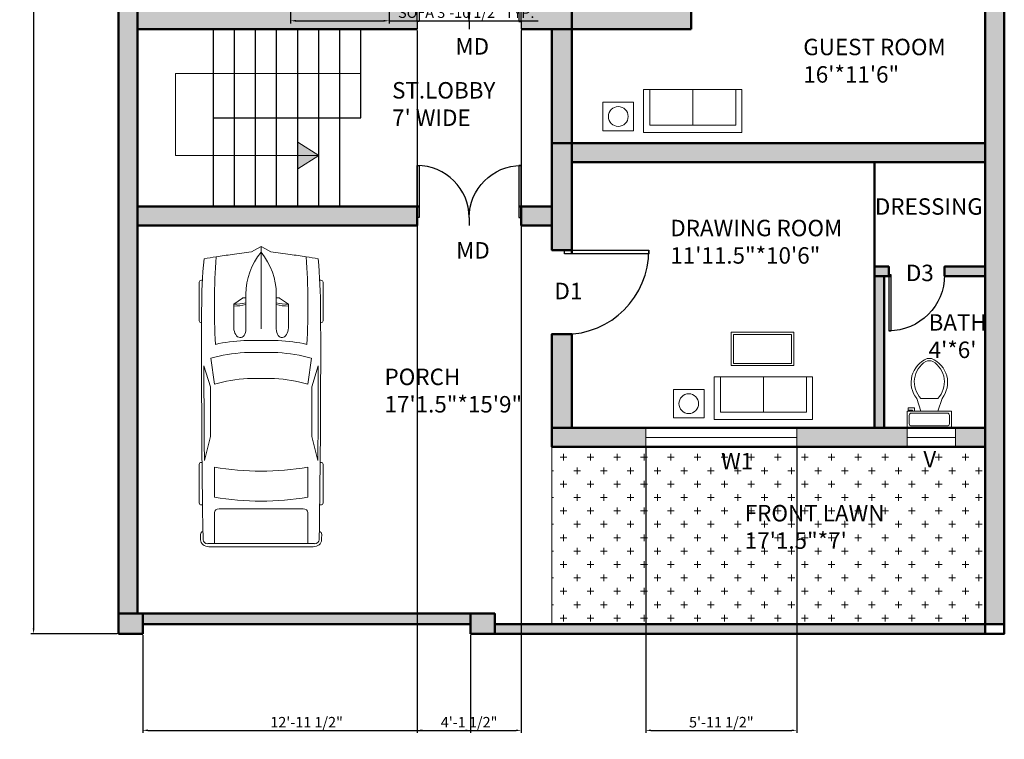
# Model space of a CAD drawing. Units: inches. Extents: x 2191 to 2715, y 2502 to 3448.
# Tile 1 of 3: x 2201 to 2668, y 2502 to 2843. Entities that reach past the tile are written whole.
import ezdxf

# ---------------------------------------------------------------- set-up
doc = ezdxf.new("R2010")
doc.units = ezdxf.units.IN
for name, color, linetype, lineweight in [('A-ANNO-DIMS', 2, 'Continuous', 18), ('A-ANNO-SYMB', 7, 'Continuous', 18), ('A-AREA-IDEN', 130, 'Continuous', 25), ('A-FLOR-FIXT', 8, 'Continuous', 18), ('A-FLOR-STRS', 7, 'Continuous', 25), ('A-WALL-PATT', 150, 'Continuous', 13), ('C-VEHI', 8, 'Continuous', 13), ('DOOR', 52, 'Continuous', 25), ('FUR', 140, 'Continuous', 18), ('L-PLNT', 3, 'Continuous', 18), ('L-PLNT-PATT', 9, 'Continuous', 13), ('TEXT', 130, 'Continuous', 18), ('WALL', 150, 'Continuous', 50), ('WIN', 210, 'Continuous', 18)]:
    doc.layers.add(name, color=color, linetype=linetype, lineweight=lineweight)
doc.styles.get("Standard").update_dxf_attribs({"font": 'arial.ttf'})
doc.dimstyles.new('ISO-25', dxfattribs={"dimtxt": 5, "dimasz": 2.5, "dimexe": 1.25, "dimexo": 0.625, "dimtad": 1, "dimdec": 0, "dimlunit": 4, "dimtxsty": 'Standard', "dimcen": 2.5, "dimadec": 0, "dimazin": 0, "dimtfac": 1, "dimtdec": 0, "dimtmove": 0, "dimatfit": 3, "dimfxl": 1, "dimarcsym": 0})

# ---------------------------------------------------------------- blocks, each defined once
blk = doc.blocks.new('*U7')
for p, q in [((21.1, 37.41), (21.1, 36.83)), ((46.55, 38.89), (22.35, 38.89)), ((47.8, 37.39), (47.8, 37.41)), ((135.45, 37.07), (135.45, 37.41)), ((136.7, 38.89), (160.9, 38.89)), ((162.15, 37.41), (162.15, 36.77)), ((70.03, 31.54), (86.41, 29.35)), ((87.99, 31.87), (74.76, 35.92)), ((134.31, 35.6), (119.29, 31.78)), ((186.47, -33.5), (186.47, 33.5)), ((188.4, -32.76), (188.4, 32.76)), ((138.42, 29.35), (157.25, 29.35)), ((164.52, 26.39), (164.52, -26.39)), ((186.47, 29.35), (167.01, 29.35)), ((32.27, 11.63), (36.13, 17.17)), ((36.13, 17.17), (50.94, 17.17)), ((29.77, 9.51), (51.68, 9.51)), ((32.12, 9.51), (32.12, 11.15)), ((58.92, -10.77), (58.92, 10.77)), ((66.55, -10.53), (66.55, 10.53)), ((82.74, 8.5), (82.74, -8.5)), ((186.47, -10.53), (186.47, 10.53)), ((3.27, 6.13), (0.1, 0.41)), ((0, 0), (51.68, 0)), ((0.1, -0.41), (3.27, -6.13)), ((29.77, -9.51), (51.68, -9.51)), ((32.12, -9.51), (32.12, -11.15)), ((32.27, -11.63), (36.13, -17.17)), ((36.13, -17.17), (50.94, -17.17)), ((86.41, -29.35), (70.03, -31.54)), ((157.25, -29.35), (138.42, -29.35)), ((167.01, -29.35), (186.47, -29.35)), ((21.1, -37.41), (21.1, -36.83)), ((87.99, -31.87), (74.76, -35.92)), ((134.31, -35.6), (119.29, -31.78)), ((135.45, -37.07), (135.45, -37.41)), ((162.15, -37.41), (162.15, -36.77)), ((46.55, -38.89), (22.35, -38.89)), ((47.8, -37.39), (47.8, -37.41)), ((136.7, -38.89), (160.9, -38.89))]:
    blk.add_line(p, q)
for centre, major_axis, ratio, start_param, end_param in [((41.19, -490.86), (0, 528.23), 0.842304, 0.00281, 0.075598), ((22.35, 37.41), (0, -1.48), 0.842304, 3.141593, 4.712389), ((64.48, -10555.62), (0, 10593.03), 0.842304, -0.013397, 0.002797), ((46.55, 37.41), (0, 1.48), 0.842304, -1.570796, 0), ((136.7, 37.41), (0, -1.48), 0.842304, 3.141593, 4.712389), ((160.9, 37.41), (0, 1.48), 0.842304, -1.570796, 0), ((180.63, 35.84), (0, 2.22), 0.842304, -0.013017, 1.249894), ((64.48, -10556.36), (0, 10595.31), 0.842304, -0.013397, -0.013017), ((183.98, 32.76), (0, -5.25), 0.842304, 1.570796, 3.128196), ((266.03, -27.52), (0, 313.31), 0.842304, 1.367076, 1.39176), ((135.29, 5.39), (0, 81.77), 0.842304, 1.245306, 1.50788), ((64.48, -10555.62), (0, -10591.55), 0.842304, 3.133765, 3.140441), ((95.79, -3666.35), (0, -3698.24), 0.842304, 3.134049, 3.144098), ((183.98, 33.5), (0, -2.96), 0.842304, 1.570796, 3.128196), ((259.18, -27.52), (0, -305.3), 0.842304, 4.528606, 4.561838), ((37.47, -593.96), (0, -623.33), 0.842304, 3.096046, 3.200911), ((134.4, 5.39), (0, -89.78), 0.842304, 4.449482, 4.652344), ((149.6, 2.8), (0, -79.58), 0.842304, 4.372215, 4.640744), ((17.08, 0), (0, 147.02), 0.842304, 4.511394, 4.913384), ((35.91, 0), (0, 147.02), 0.842304, 4.511394, 4.913384), ((167.01, 26.39), (0, 2.96), 0.842304, 0, 1.570796), ((-204.49, 52.4), (0, -250.96), 0.842304, 1.385369, 1.434372), ((13.04, 17.01), (0, 27.42), 0.842304, 4.435146, 4.718221), ((14.2, 17.01), (0, 27.42), 0.842304, 4.435146, 4.718221), ((50.79, 13.34), (6.34, -0.36), 0.603834, -1.395552, 1.581315), ((29.77, -46.66), (0, 56.17), 0.842304, 0, 0.590319), ((32.75, 11.15), (0, 0.74), 0.842304, 0.879714, 1.570796), ((0.62, 0), (0, -0.74), 0.842304, 4.131459, 5.293319), ((-204.49, -52.4), (0, 250.96), 0.842304, -1.434372, -1.385369), ((29.77, 46.66), (0, 56.17), 0.842304, 2.551274, 3.141593), ((32.75, -11.15), (0, -0.74), 0.842304, 4.712389, 5.403472), ((13.04, -17.01), (0, -27.42), 0.842304, 1.564964, 1.848039), ((14.2, -17.01), (0, -27.42), 0.842304, 1.564964, 1.848039), ((134.4, -5.39), (0, -89.78), 0.842304, -1.510751, -1.307889), ((135.29, -5.39), (0, -81.77), 0.842304, -1.50788, -1.245306), ((149.6, -2.8), (0, -79.58), 0.842304, -1.499151, -1.230623), ((259.18, 27.52), (0, 305.3), 0.842304, 1.721348, 1.754579), ((266.03, 27.52), (0, 313.31), 0.842304, 1.749832, 1.774517), ((37.47, 593.96), (0, -623.33), 0.842304, -0.059319, 0.045547), ((167.01, -26.39), (0, -2.96), 0.842304, 4.712389, 6.283185), ((41.19, 490.86), (0, -528.23), 0.842304, -0.075598, -0.00281), ((64.48, 10555.62), (0, 10593.03), 0.842304, 3.138796, 3.15499), ((64.48, 10555.62), (0, -10591.55), 0.842304, 0.001152, 0.007828), ((95.79, 3666.35), (0, -3698.24), 0.842304, -0.002505, 0.007544), ((180.63, -35.84), (0, -2.22), 0.842304, -1.249894, 0.013017), ((183.98, -33.5), (0, 2.96), 0.842304, 3.15499, 4.712389), ((183.98, -32.76), (0, -5.25), 0.842304, 0.013397, 1.570796), ((22.35, -37.41), (0, 1.48), 0.842304, 1.570796, 3.141593), ((46.55, -37.41), (0, -1.48), 0.842304, 0, 1.570796), ((136.7, -37.41), (0, -1.48), 0.842304, -1.570796, 0), ((160.9, -37.41), (0, 1.48), 0.842304, 3.141593, 4.712389), ((64.48, 10556.36), (0, 10595.31), 0.842304, 3.15461, 3.15499)]:
    blk.add_ellipse(centre, major_axis=major_axis, ratio=ratio, start_param=start_param, end_param=end_param)
at = {"extrusion": (0, 0, -1)}
blk.add_ellipse((50.79, -13.34), major_axis=(6.34, 0.36), ratio=0.603834, start_param=-1.395552, end_param=1.581315, dxfattribs=at)
blk = doc.blocks.new('*U2')
for p, q in [((0, 0), (0, -6)), ((40, 0), (40, -6))]:
    blk.add_line(p, q)
blk.add_lwpolyline([(0, 0), (0, 40), (1.75, 40), (1.75, 0)], close=True)
blk.add_arc((0, 0), 40, 0, 90)
blk = doc.blocks.new('*U4')
for p, q in [((9.5, -6), (9.5, -2)), ((-10, -8.5), (-8, -8.5)), ((-10, -9.5), (-10, -8.5)), ((-8, -8.5), (-8, -8)), ((-7, -8), (-7, -9.5)), ((-4, -8), (-6, -14)), ((4, -8), (6, -14)), ((-7, -9.5), (-10, -9.5)), ((4, -14), (-4, -14))]:
    blk.add_line(p, q)
blk.add_lwpolyline([(10.5, -8), (10.5, 0), (-10.5, 0), (-10.5, -8)], close=True)
for points in [[(-9.5, -2), (-9.5, -6)], [(8.5, -1), (-8.5, -1)], [(-8.5, -7), (8.5, -7)]]:
    blk.add_lwpolyline(points)
for centre, radius, start, end in [((-8.62, -1.88), 0.884, 81.8699, 188.1301), ((8.62, -1.88), 0.884, 351.8699, 98.1301), ((-8.62, -6.12), 0.884, 171.8699, 278.1301), ((8.62, -6.12), 0.884, 261.8699, 8.1301), ((3.52, -21.58), 12.17, 141.4691, 247.9714), ((4.2, -21.82), 11.33, 136.3677, 238.9468), ((-3.52, -21.58), 12.17, 292.0284, 38.5307), ((-4.2, -21.82), 11.33, 301.053, 43.6321), ((0, -27.88), 4, 245.7318, 294.2682), ((0, -29), 4, 254.8605, 285.1395)]:
    blk.add_arc(centre, radius, start, end)
blk = doc.blocks.new('*D9')
at = {"layer": 'A-ANNO-DIMS', "color": 0, "lineweight": -2, "transparency": 16777216}
for p, q in [((2247.34, 3391.65), (2206.49, 3391.65)), ((2207.74, 3389.15), (2207.74, 2554.15)), ((2247.34, 2551.65), (2206.49, 2551.65))]:
    blk.add_line(p, q, dxfattribs=at)
at = {"layer": 'A-ANNO-DIMS', "color": 0, "lineweight": 100, "transparency": 16777216}
for points in [[(2207.32, 3389.15), (2208.15, 3389.15), (2207.74, 3391.65)], [(2207.32, 2554.15), (2208.15, 2554.15), (2207.74, 2551.65)]]:
    blk.add_solid(points, dxfattribs=at)
at = {"layer": 'Defpoints', "color": 0, "lineweight": 100, "transparency": 16777216}
for p in [(2247.96, 3391.65), (2207.74, 2551.65), (2247.96, 2551.65)]:
    blk.add_point(p, dxfattribs=at)
at = {"layer": 'A-ANNO-DIMS', "color": 0, "transparency": 16777216, "insert": (2204.56, 2971.65), "char_height": 5, "attachment_point": 5, "rotation": 90}
blk.add_mtext("70'", dxfattribs=at)
blk = doc.blocks.new('SOFA-TWO-SEAT')
for p, q in [((3.01, 20.24), (0, 20.24)), ((0, 20.24), (0, 0)), ((23.39, 20.24), (23.39, 3.45)), ((43.77, 20.24), (46.65, 20.24)), ((46.65, 20.24), (46.65, 20.24)), ((46.65, 20.24), (46.65, 0)), ((0, 0), (46.65, 0))]:
    blk.add_line(p, q)
blk.add_lwpolyline([(43.77, 3.45), (3.01, 3.45), (3.01, 20.24), (43.77, 20.24)], close=True)
blk = doc.blocks.new('TABLE-END-ROUND-ON-SQUARE')
blk.add_lwpolyline([(14.61, 0), (0, 0), (0, 13.55), (14.61, 13.55)], close=True)
blk.add_circle((7.31, 6.78), 4.68)
blk = doc.blocks.new('*D16')
at = {"layer": 'A-ANNO-DIMS', "color": 0, "lineweight": -2, "transparency": 16777216}
for p, q in [((2329.62, 2848.52), (2329.62, 2840.89)), ((2376.27, 2848.52), (2376.27, 2840.89)), ((2332.12, 2842.14), (2373.77, 2842.14)), ((2376.27, 2842.14), (2446.96, 2842.14))]:
    blk.add_line(p, q, dxfattribs=at)
at = {"layer": 'A-ANNO-DIMS', "color": 0, "lineweight": 100, "transparency": 16777216}
for points in [[(2332.12, 2842.56), (2332.12, 2841.73), (2329.62, 2842.14)], [(2373.77, 2842.56), (2373.77, 2841.73), (2376.27, 2842.14)]]:
    blk.add_solid(points, dxfattribs=at)
at = {"layer": 'Defpoints', "color": 0, "lineweight": 100, "transparency": 16777216}
for p in [(2329.62, 2849.14), (2376.27, 2849.14), (2376.27, 2842.14)]:
    blk.add_point(p, dxfattribs=at)
at = {"layer": 'A-ANNO-DIMS', "color": 0, "transparency": 16777216, "insert": (2412.87, 2845.36), "char_height": 5, "attachment_point": 5}
blk.add_mtext('SOFA 3\'-10 1/2" TYP.', dxfattribs=at)
blk = doc.blocks.new('*D30')
at = {"layer": 'A-ANNO-DIMS', "color": 0, "lineweight": -2, "transparency": 16777216}
for p, q in [((2389.52, 2837.53), (2389.52, 2504.6)), ((2438.92, 2837.53), (2438.92, 2504.6)), ((2392.02, 2505.85), (2436.42, 2505.85))]:
    blk.add_line(p, q, dxfattribs=at)
at = {"layer": 'A-ANNO-DIMS', "color": 0, "lineweight": 100, "transparency": 16777216}
for points in [[(2392.02, 2506.27), (2392.02, 2505.44), (2389.52, 2505.85)], [(2436.42, 2506.27), (2436.42, 2505.44), (2438.92, 2505.85)]]:
    blk.add_solid(points, dxfattribs=at)
at = {"layer": 'Defpoints', "color": 0, "lineweight": 100, "transparency": 16777216}
for p in [(2389.52, 2838.15), (2438.92, 2838.15), (2438.92, 2505.85)]:
    blk.add_point(p, dxfattribs=at)
at = {"layer": 'A-ANNO-DIMS', "color": 0, "transparency": 16777216, "insert": (2414.22, 2509.06), "char_height": 5, "attachment_point": 5}
blk.add_mtext('4\'-1 1/2"', dxfattribs=at)
blk = doc.blocks.new('*D36')
at = {"layer": 'A-ANNO-DIMS', "color": 0, "lineweight": -2, "transparency": 16777216}
for p, q in [((2259.47, 2551.03), (2259.47, 2504.6)), ((2414.87, 2551.03), (2414.87, 2504.6)), ((2261.97, 2505.85), (2412.37, 2505.85))]:
    blk.add_line(p, q, dxfattribs=at)
at = {"layer": 'A-ANNO-DIMS', "color": 0, "lineweight": 100, "transparency": 16777216}
for points in [[(2261.97, 2506.27), (2261.97, 2505.44), (2259.47, 2505.85)], [(2412.37, 2506.27), (2412.37, 2505.44), (2414.87, 2505.85)]]:
    blk.add_solid(points, dxfattribs=at)
at = {"layer": 'Defpoints', "color": 0, "lineweight": 100, "transparency": 16777216}
for p in [(2259.47, 2551.65), (2414.87, 2551.65), (2414.87, 2505.85)]:
    blk.add_point(p, dxfattribs=at)
at = {"layer": 'A-ANNO-DIMS', "color": 0, "transparency": 16777216, "insert": (2337.17, 2509.06), "char_height": 5, "attachment_point": 5}
blk.add_mtext('12\'-11 1/2"', dxfattribs=at)
blk = doc.blocks.new('*D37')
at = {"layer": 'A-ANNO-DIMS', "color": 0, "lineweight": -2, "transparency": 16777216}
for p, q in [((2497.99, 2639.53), (2497.99, 2504.6)), ((2569.61, 2639.53), (2569.61, 2504.6)), ((2500.49, 2505.85), (2567.11, 2505.85))]:
    blk.add_line(p, q, dxfattribs=at)
at = {"layer": 'A-ANNO-DIMS', "color": 0, "lineweight": 100, "transparency": 16777216}
for points in [[(2500.49, 2506.27), (2500.49, 2505.44), (2497.99, 2505.85)], [(2567.11, 2506.27), (2567.11, 2505.44), (2569.61, 2505.85)]]:
    blk.add_solid(points, dxfattribs=at)
at = {"layer": 'Defpoints', "color": 0, "lineweight": 100, "transparency": 16777216}
for p in [(2497.99, 2640.15), (2569.61, 2640.15), (2569.61, 2505.85)]:
    blk.add_point(p, dxfattribs=at)
at = {"layer": 'A-ANNO-DIMS', "color": 0, "transparency": 16777216, "insert": (2533.8, 2509.06), "char_height": 5, "attachment_point": 5}
blk.add_mtext('5\'-11 1/2"', dxfattribs=at)

msp = doc.modelspace()

# ---------------------------------------------------------------- hatches: boundary and pattern name
at = {"layer": 'A-ANNO-SYMB'}
h = msp.add_hatch(color=256, dxfattribs=at)
h.dxf.hatch_style = 1
h.paths.add_polyline_path([(2332.96, 2784.6), (2332.96, 2778.31), (2342.96, 2778.31)])
h.paths.add_polyline_path([(2342.96, 2778.31), (2332.96, 2778.31), (2332.96, 2772.02)])
at = {"layer": 'A-WALL-PATT'}
h = msp.add_hatch(color=256, dxfattribs=at)
h.dxf.hatch_style = 1
h.paths.add_polyline_path([(2658.96, 3391.65), (2247.96, 3391.65), (2247.96, 3382.65), (2658.96, 3382.65)])
h.paths.add_polyline_path([(2256.96, 3382.65), (2247.96, 3382.65), (2247.96, 2561.19), (2256.96, 2561.19)])
h.paths.add_polyline_path([(2316.96, 3382.65), (2312.46, 3382.65), (2312.46, 3318.18), (2316.96, 3318.18)])
h.paths.add_polyline_path([(2412.96, 3279.15), (2308.33, 3279.15), (2308.33, 3270.15), (2412.96, 3270.15)])
h.paths.add_polyline_path([(2263, 3279.15), (2256.96, 3279.15), (2256.96, 3270.15), (2263, 3270.15)])
h.paths.add_polyline_path([(2421.96, 3323.7), (2412.96, 3323.7), (2412.96, 3279.15), (2421.96, 3279.15)])
h.paths.add_polyline_path([(2421.96, 3382.65), (2412.96, 3382.65), (2412.96, 3366.03), (2421.96, 3366.03)])
h.paths.add_polyline_path([(2421.96, 3279.15), (2412.96, 3279.15), (2412.96, 3270.15), (2412.96, 3120.46), (2421.96, 3120.46)])
h.paths.add_polyline_path([(2469.63, 3310.65), (2421.96, 3310.65), (2421.96, 3301.65), (2469.63, 3301.65)])
h.paths.add_polyline_path([(2594.46, 3310.65), (2549.09, 3310.65), (2549.09, 3301.65), (2594.46, 3301.65)])
h.paths.add_polyline_path([(2658.96, 3298.65), (2632.95, 3298.65), (2632.95, 3294.15), (2658.96, 3294.15)])
h.paths.add_polyline_path([(2600.93, 3298.65), (2598.96, 3298.65), (2598.96, 3328.67), (2594.46, 3328.67), (2594.46, 3310.65), (2594.46, 3294.15), (2594.46, 3284.36), (2598.96, 3284.36), (2598.96, 3294.15), (2600.93, 3294.15)])
h.paths.add_polyline_path([(2598.96, 3382.65), (2594.46, 3382.65), (2594.46, 3368.86), (2598.96, 3368.86), (2598.96, 3369.76)])
h.paths.add_polyline_path([(2667.96, 3391.65), (2658.96, 3391.65), (2658.96, 3382.65), (2658.96, 2551.65), (2667.96, 2551.65)])
h.paths.add_polyline_path([(2414.87, 2561.19), (2259.47, 2561.19), (2259.47, 2556.15), (2414.87, 2556.15)])
h.paths.add_polyline_path([(2259.47, 2561.19), (2247.96, 2561.19), (2247.96, 2551.65), (2259.47, 2551.65)])
h.paths.add_polyline_path([(2426.37, 2561.19), (2414.87, 2561.19), (2414.87, 2556.15), (2414.87, 2551.65), (2426.37, 2551.65), (2426.37, 2556.15)])
h.paths.add_polyline_path([(2667.96, 2556.15), (2426.37, 2556.15), (2426.37, 2551.65), (2667.96, 2551.65)])
h.paths.add_polyline_path([(2497.99, 2649.15), (2453.46, 2649.15), (2453.46, 2640.15), (2497.99, 2640.15)])
h.paths.add_polyline_path([(2462.96, 2693.64), (2453.46, 2693.64), (2453.46, 2649.15), (2462.96, 2649.15)])
h.paths.add_polyline_path([(2621.93, 2649.15), (2569.61, 2649.15), (2569.61, 2640.15), (2621.93, 2640.15)])
h.paths.add_polyline_path([(2610.96, 2721.15), (2606.46, 2721.15), (2606.46, 2649.15), (2610.96, 2649.15)])
h.paths.add_polyline_path([(2658.96, 2649.15), (2644.82, 2649.15), (2644.82, 2640.15), (2658.96, 2640.15)])
h.paths.add_polyline_path([(2462.96, 2784.15), (2453.46, 2784.15), (2453.46, 2733.49), (2459.46, 2733.49), (2462.96, 2733.49)])
h.paths.add_polyline_path([(2453.46, 2754.15), (2438.92, 2754.15), (2438.92, 2748.86), (2438.92, 2745.15), (2453.46, 2745.15)])
h.paths.add_polyline_path([(2389.52, 2754.15), (2256.96, 2754.15), (2256.96, 2745.15), (2389.52, 2745.15), (2389.52, 2748.86)])
h.paths.add_polyline_path([(2658.96, 2784.15), (2462.96, 2784.15), (2462.96, 2775.15), (2658.96, 2775.15)])
h.paths.add_polyline_path([(2658.96, 2725.65), (2639.65, 2725.65), (2639.65, 2721.68, -0.005), (2639.64, 2721.15), (2658.96, 2721.15)])
h.paths.add_polyline_path([(2613.17, 2725.65), (2606.46, 2725.65), (2606.46, 2721.15), (2610.96, 2721.15), (2613.17, 2721.15), (2613.17, 2721.68)])
h.paths.add_polyline_path([(2462.96, 2838.15), (2453.46, 2838.15), (2453.46, 2784.15), (2462.96, 2784.15)])
h.paths.add_polyline_path([(2389.52, 2847.15), (2256.96, 2847.15), (2256.96, 2838.15), (2389.52, 2838.15), (2389.52, 2841.86)])
h.paths.add_polyline_path([(2307.96, 2890.63), (2298.96, 2890.63), (2298.96, 2847.15), (2307.96, 2847.15)])
h.paths.add_polyline_path([(2462.96, 2847.15), (2453.96, 2847.15), (2438.92, 2847.15), (2438.92, 2841.86), (2438.92, 2838.15), (2453.96, 2838.15), (2462.96, 2838.15)])
h.paths.add_polyline_path([(2519.46, 2873.86, -0.01877), (2516.46, 2873.75), (2510.46, 2873.75), (2510.46, 2847.15), (2462.96, 2847.15), (2462.96, 2838.15), (2519.46, 2838.15)])
h.paths.add_polyline_path([(2519.46, 2922.15), (2510.46, 2922.15), (2510.46, 2913.75), (2516.46, 2913.75), (2519.46, 2913.75)])
h.paths.add_polyline_path([(2519.46, 2991.15), (2519.46, 3078.15), (2510.46, 3078.15), (2510.46, 3069.15), (2510.46, 2931.15), (2510.46, 2922.15), (2519.46, 2922.15), (2519.46, 2928.9), (2519.46, 2931.15)])
h.paths.add_polyline_path([(2609.08, 2926.65), (2556.08, 2926.65), (2556.08, 2922.15), (2609.08, 2922.15)])
h.paths.add_polyline_path([(2658.96, 2926.65), (2648.34, 2926.65), (2648.34, 2922.15), (2656.8, 2922.15), (2658.96, 2922.15)])
h.paths.add_polyline_path([(2603.46, 2931.15), (2603.46, 2935.9), (2598.96, 2935.9), (2598.96, 2931.15), (2598.96, 2926.65), (2603.46, 2926.65)])
h.paths.add_polyline_path([(2609.35, 3000.15), (2603.46, 3000.15), (2519.46, 3000.15), (2519.46, 2991.15), (2598.96, 2991.15), (2598.96, 2980.21), (2603.46, 2980.21), (2603.46, 2991.15), (2609.35, 2991.15)])
h.paths.add_polyline_path([(2658.96, 3000.15), (2649.75, 3000.15), (2649.75, 2991.15), (2658.96, 2991.15)])
h.paths.add_polyline_path([(2307.96, 2977.56), (2298.96, 2977.56), (2298.96, 2951.93), (2307.96, 2951.93)])
h.paths.add_polyline_path([(2307.96, 3069.15), (2298.96, 3069.15), (2298.96, 3038.86), (2307.96, 3038.86)])
h.paths.add_polyline_path([(2510.46, 3078.15), (2298.96, 3078.15), (2298.96, 3069.15), (2307.96, 3069.15), (2510.46, 3069.15)])
h.paths.add_polyline_path([(2421.96, 3080.46), (2415.96, 3080.46), (2412.96, 3080.46), (2412.96, 3078.15), (2421.96, 3078.15)])
h.paths.add_polyline_path([(2519.46, 3083.52, -0.01877), (2516.46, 3083.41), (2510.46, 3083.41), (2510.46, 3078.15), (2519.46, 3078.15)])
h.paths.add_polyline_path([(2519.46, 3127.65), (2510.46, 3127.65), (2510.46, 3123.41), (2516.46, 3123.41), (2519.46, 3123.41)])
h.paths.add_polyline_path([(2427.29, 3133.65), (2427.29, 3136.65), (2421.96, 3136.65), (2421.96, 3127.65), (2427.29, 3127.65)])
h.paths.add_polyline_path([(2598.96, 3136.65), (2467.29, 3136.65), (2467.29, 3127.65), (2598.96, 3127.65)])
h.paths.add_polyline_path([(2316.96, 3285.93), (2312.46, 3285.93), (2312.46, 3279.15), (2316.96, 3279.15)])
h.paths.add_polyline_path([(2658.96, 3234.15), (2598.96, 3234.15), (2598.96, 3229.65), (2658.96, 3229.65)])
h.paths.add_polyline_path([(2598.96, 3241.45), (2594.46, 3241.45), (2594.46, 3136.65), (2598.96, 3136.65)])
h.paths.add_polyline_path([(2658.96, 3136.65), (2632.67, 3136.65), (2632.67, 3127.65), (2658.96, 3127.65)])
h.paths.add_polyline_path([(2600.93, 3132.46), (2600.93, 3136.65), (2598.96, 3136.65), (2598.96, 3127.65), (2600.93, 3127.65)])
h.paths.add_polyline_path([(2524.07, 2926.65), (2519.46, 2926.65), (2519.46, 2922.15), (2524.07, 2922.15)])
at = {"layer": 'L-PLNT-PATT'}
h = msp.add_hatch(dxfattribs=at)
h.set_pattern_fill('CROSS', color=256)
h.paths.add_polyline_path([(2658.96, 2640.15), (2453.46, 2640.15), (2453.46, 2556.15), (2658.96, 2556.15)])

# ---------------------------------------------------------------- linework, layer by layer
at = {"layer": 'A-ANNO-SYMB'}
for p, q in [((2362.96, 2817.15), (2274.99, 2817.15)), ((2274.99, 2817.15), (2274.99, 2778.31)), ((2342.96, 2778.31), (2332.96, 2784.6)), ((2274.99, 2778.31), (2342.96, 2778.31)), ((2342.96, 2778.31), (2332.96, 2772.02))]:
    msp.add_line(p, q, dxfattribs=at)
at = {"layer": 'A-FLOR-STRS'}
for p, q in [((2292.96, 2754.15), (2292.96, 2838.15)), ((2302.96, 2754.15), (2302.96, 2838.15)), ((2312.96, 2754.15), (2312.96, 2838.15)), ((2322.96, 2754.15), (2322.96, 2838.15)), ((2332.96, 2754.15), (2332.96, 2838.15)), ((2342.96, 2754.15), (2342.96, 2838.15)), ((2352.96, 2754.15), (2352.96, 2838.15)), ((2362.96, 2796.15), (2362.96, 2838.15)), ((2292.96, 2796.15), (2355.58, 2796.15)), ((2355.58, 2796.15), (2362.96, 2796.15)), ((2256.96, 2754.15), (2292.96, 2754.15))]:
    msp.add_line(p, q, dxfattribs=at)
at = {"layer": 'FUR'}
for points in [[(2538.54, 2678.77), (2568.14, 2678.77), (2568.14, 2694.53), (2538.54, 2694.53)], [(2539.54, 2679.77), (2567.14, 2679.77), (2567.14, 2693.53), (2539.54, 2693.53)]]:
    msp.add_lwpolyline(points, close=True, dxfattribs=at)
at = {"layer": 'L-PLNT'}
msp.add_line((2453.46, 2556.15), (2453.46, 2640.15), dxfattribs=at)
msp.add_line((2453.46, 2556.15), (2453.46, 2640.15), dxfattribs=at)
at = {"layer": 'WALL'}
for p, q in [((2247.96, 2551.65), (2247.96, 3391.65)), ((2667.96, 3391.65), (2667.96, 2551.65)), ((2256.96, 2561.19), (2256.96, 3382.65)), ((2658.96, 3382.65), (2658.96, 2551.65)), ((2658.96, 2784.15), (2658.96, 2922.15)), ((2519.46, 2873.86), (2519.46, 2838.15)), ((2462.96, 2784.15), (2462.96, 2847.15)), ((2256.96, 2754.15), (2256.96, 2838.15)), ((2256.96, 2838.15), (2389.52, 2838.15)), ((2438.92, 2838.15), (2453.96, 2838.15)), ((2453.46, 2784.15), (2453.46, 2838.15)), ((2453.96, 2838.15), (2519.46, 2838.15)), ((2453.46, 2784.15), (2606.46, 2784.15)), ((2453.46, 2733.49), (2453.46, 2784.15)), ((2462.96, 2775.15), (2462.96, 2784.15)), ((2606.46, 2784.15), (2658.96, 2784.15)), ((2462.96, 2775.15), (2606.46, 2775.15)), ((2462.96, 2731.74), (2462.96, 2775.15)), ((2606.46, 2775.15), (2606.46, 2725.65)), ((2606.46, 2775.15), (2658.96, 2775.15)), ((2256.96, 2754.15), (2390.6, 2754.15)), ((2437.84, 2754.15), (2453.46, 2754.15)), ((2256.96, 2561.19), (2256.96, 2745.15)), ((2256.96, 2745.15), (2389.52, 2745.15)), ((2438.92, 2745.15), (2453.46, 2745.15)), ((2606.46, 2725.65), (2606.46, 2649.15)), ((2613.17, 2725.65), (2606.46, 2725.65)), ((2658.96, 2725.65), (2639.65, 2725.65)), ((2610.96, 2721.15), (2610.96, 2649.15)), ((2614.33, 2721.15), (2610.96, 2721.15)), ((2658.96, 2721.15), (2639.64, 2721.15)), ((2658.96, 2649.15), (2658.96, 2721.15)), ((2462.96, 2649.15), (2462.96, 2693.64)), ((2462.96, 2649.15), (2462.96, 2693.64)), ((2453.46, 2649.15), (2453.46, 2693.49)), ((2453.46, 2649.15), (2658.96, 2649.15)), ((2453.46, 2640.15), (2453.46, 2649.15)), ((2606.46, 2649.15), (2462.96, 2649.15)), ((2453.46, 2640.15), (2658.96, 2640.15)), ((2667.96, 2556.15), (2426.37, 2556.15)), ((2658.96, 2556.15), (2453.46, 2556.15)), ((2259.47, 2551.65), (2247.96, 2551.65)), ((2667.96, 2551.65), (2414.87, 2551.65))]:
    msp.add_line(p, q, dxfattribs=at)
for points in [[(2658.96, 3391.65), (2667.96, 3391.65), (2667.96, 2551.65), (2658.96, 2551.65)], [(2247.96, 2561.19), (2256.96, 2561.19), (2256.96, 3382.65), (2247.96, 3382.65)], [(2453.46, 2838.15), (2462.96, 2838.15), (2462.96, 2784.15), (2453.46, 2784.15)], [(2453.46, 2784.15), (2462.96, 2784.15), (2462.96, 2733.49), (2453.46, 2733.49)], [(2658.96, 2775.15), (2462.96, 2775.15), (2462.96, 2784.15), (2658.96, 2784.15)], [(2658.96, 2775.15), (2658.96, 2775.15), (2658.96, 2775.15), (2658.96, 2775.15)], [(2256.96, 2745.15), (2389.52, 2745.15), (2389.52, 2754.15), (2256.96, 2754.15)], [(2438.92, 2745.15), (2453.46, 2745.15), (2453.46, 2754.15), (2438.92, 2754.15)], [(2606.46, 2725.65), (2613.17, 2725.65), (2613.17, 2721.15), (2606.46, 2721.15)], [(2639.64, 2721.15), (2658.96, 2721.15), (2658.96, 2725.65), (2639.64, 2725.65)], [(2606.46, 2721.15), (2610.96, 2721.15), (2610.96, 2649.15), (2606.46, 2649.15)], [(2453.46, 2649.15), (2462.96, 2649.15), (2462.96, 2693.64), (2453.46, 2693.64)], [(2247.96, 2551.65), (2259.47, 2551.65), (2259.47, 2561.19), (2247.96, 2561.19)], [(2414.87, 2561.19), (2259.47, 2561.19), (2259.47, 2556.15), (2414.87, 2556.15)], [(2414.87, 2551.65), (2426.37, 2551.65), (2426.37, 2561.19), (2414.87, 2561.19)], [(2426.37, 2556.15), (2667.96, 2556.15), (2667.96, 2556.15), (2426.37, 2556.15)], [(2426.37, 2551.65), (2667.96, 2551.65), (2667.96, 2556.15), (2426.37, 2556.15)]]:
    msp.add_lwpolyline(points, close=True, dxfattribs=at)
for points in [[(2497.99, 2649.15), (2453.46, 2649.15), (2453.46, 2640.15), (2497.99, 2640.15)], [(2621.93, 2649.15), (2569.61, 2649.15)], [(2644.82, 2640.15), (2658.96, 2640.15), (2658.96, 2649.15), (2642.93, 2649.15)], [(2569.61, 2640.15), (2621.93, 2640.15)]]:
    msp.add_lwpolyline(points, dxfattribs=at)
at = {"layer": 'WIN'}
for p, q in [((2621.93, 2649.15), (2644.82, 2649.15)), ((2497.99, 2644.65), (2569.61, 2644.65)), ((2621.93, 2644.65), (2644.82, 2644.65))]:
    msp.add_line(p, q, dxfattribs=at)
for points in [[(2497.99, 2649.15), (2569.61, 2649.15), (2569.61, 2640.15), (2497.99, 2640.15)], [(2621.93, 2649.15), (2644.82, 2649.15), (2644.82, 2640.15), (2621.93, 2640.15)]]:
    msp.add_lwpolyline(points, close=True, dxfattribs=at)

# ---------------------------------------------------------------- block references
at = {"layer": 'A-FLOR-FIXT', "xscale": -1, "rotation": 180}
msp.add_blockref('*U4', (2632.43, 2649.15), dxfattribs=at)
at = {"layer": 'C-VEHI', "xscale": 0.7549308442728768, "yscale": 0.7549308442728768, "zscale": 0.7549308442728768, "rotation": 270}
msp.add_blockref('*U7', (2315.61, 2735.1), dxfattribs=at)
at = {"layer": 'DOOR', "yscale": 0.617424543084726, "zscale": 0.617424543084726}
for p, xscale in [((2389.52, 2841.86), 0.617424543084726), ((2438.92, 2841.86), -0.617424543084726), ((2389.52, 2748.86), 0.617424543084726), ((2438.92, 2748.86), -0.617424543084726)]:
    msp.add_blockref('*U2', p, dxfattribs=dict(at, xscale=xscale))
at = {"layer": 'DOOR', "rotation": 270}
msp.add_blockref('*U2', (2459.46, 2733.49), dxfattribs=at)
at = {"layer": 'DOOR', "xscale": -0.6617684744906729, "yscale": 0.6617684744906729, "zscale": 0.6617684744906729, "rotation": 180}
msp.add_blockref('*U2', (2613.17, 2721.68), dxfattribs=at)
at = {"layer": 'FUR'}
for name, p in [('SOFA-TWO-SEAT', (2496.93, 2789.27)), ('TABLE-END-ROUND-ON-SQUARE', (2477.63, 2790)), ('SOFA-TWO-SEAT', (2530.37, 2653.16)), ('TABLE-END-ROUND-ON-SQUARE', (2511.06, 2653.9))]:
    msp.add_blockref(name, p, dxfattribs=at)

# ---------------------------------------------------------------- texts
at = {"layer": 'A-AREA-IDEN', "attachment_point": 1}
for s, insert, char_height in [('GUEST ROOM\\P16\'*11\'6"', (2572.67, 2833.62), 7.795), ("ST.LOBBY\\P7' WIDE", (2377.71, 2813.09), 7.795), ('DRESSING', (2606.59, 2758.02), 7.795), ('DRAWING ROOM\\P11\'11.5"*10\'6"', (2509.6, 2747.82), 7.7945), ("BATH\\P4'*6'", (2632.08, 2703.09), 7.795), ('PORCH\\P17\'1.5"*15\'9"', (2374.12, 2677.28), 7.7945), ('FRONT LAWN\\P17\'1.5"*7\'', (2544.92, 2612.67), 7.795)]:
    msp.add_mtext_dynamic_manual_height_columns(s, width=100.7314, gutter_width=38.97, heights=[0], dxfattribs=dict(at, insert=insert, char_height=char_height))
at = {"layer": 'TEXT', "attachment_point": 1}
for s, heights, insert, char_height in [('MD', [0], (2407.73, 2833.91), 7.795), ('MD', [0], (2408.07, 2737.24), 7.795), ('D3', [0], (2621.3, 2726.54), 7.795), ('D1', [0], (2454.69, 2717.97), 7.795), ('V', [0], (2629.57, 2638.3), 7.79), ('W1', [7.83], (2533.68, 2637.36), 7.795)]:
    msp.add_mtext_dynamic_manual_height_columns(s, width=100.7314, gutter_width=38.97, heights=heights, dxfattribs=dict(at, insert=insert, char_height=char_height))

# ---------------------------------------------------------------- dimensions: what is measured, and where the dimension line sits
at = {"layer": 'A-ANNO-DIMS'}
dim = msp.add_linear_dim(base=(2207.74, 2551.65), p1=(2247.96, 3391.65), p2=(2247.96, 2551.65), angle=90, dimstyle='ISO-25', override={"dimclrd": 0, "dimclre": 0, "dimclrt": 0}, dxfattribs=at)
dim.commit()
dim.dimension.update_dxf_attribs({"geometry": '*D9', "text_midpoint": (2204.56, 2971.65)})
dim = msp.add_linear_dim(base=(2376.2667, 2842.1443), p1=(2329.6151, 2849.1421), p2=(2376.2667, 2849.1421), text='SOFA <> TYP.', dimstyle='ISO-25', override={"dimdec": 1, "dimlfac": 1, "dimrnd": 0, "dimzin": 1, "dimdsep": 46, "dimlunit": 4, "dimfrac": 2}, dxfattribs=at)
dim.commit()
dim.dimension.update_dxf_attribs({"geometry": '*D16', "text_midpoint": (2412.8655, 2845.358)})
for base, p1, p2, picture, middle in [((2438.92, 2505.85), (2389.52, 2838.15), (2438.92, 2838.15), '*D30', (2414.22, 2509.06)), ((2569.61, 2505.85), (2497.99, 2640.15), (2569.61, 2640.15), '*D37', (2533.8, 2509.06)), ((2414.87, 2505.85), (2259.47, 2551.65), (2414.87, 2551.65), '*D36', (2337.17, 2509.06))]:
    dim = msp.add_linear_dim(base=base, p1=p1, p2=p2, dimstyle='ISO-25', override={"dimdec": 1, "dimlfac": 1, "dimrnd": 0, "dimzin": 1, "dimdsep": 46, "dimlunit": 4, "dimfrac": 2}, dxfattribs=at)
    dim.commit()
    dim.dimension.update_dxf_attribs({"geometry": picture, "text_midpoint": middle})

doc.saveas('drawing.dxf')
